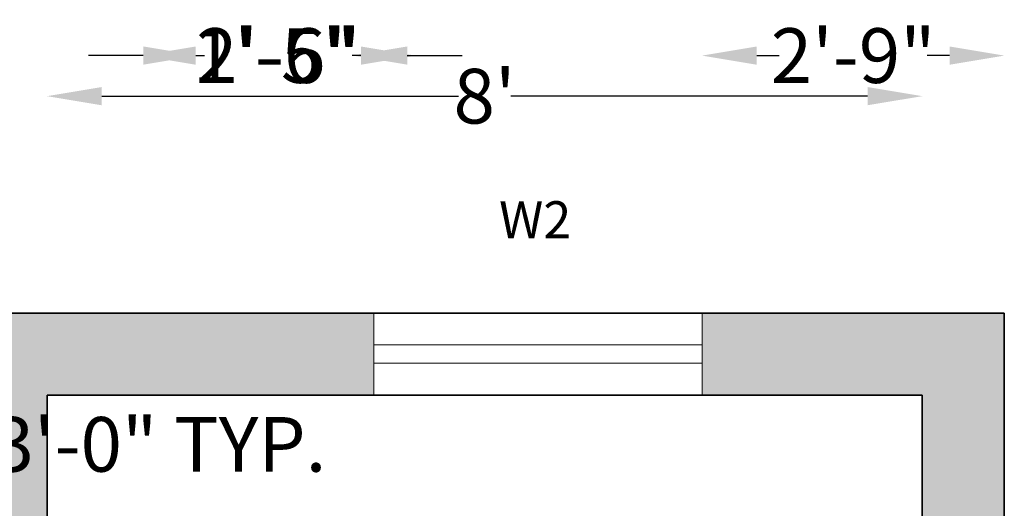
# Model space of a CAD drawing. Units: inches. Extents: x 2178 to 3409, y 1711 to 2279.
# Tile 7 of 8: x 2368 to 2476, y 2226 to 2279. Entities that reach past the tile are written whole.
import ezdxf

# ---------------------------------------------------------------- set-up
doc = ezdxf.new("R2010")
doc.units = ezdxf.units.IN
for name, color, linetype, lineweight in [('A-ANNO-DIMS', 2, 'Continuous', 18), ('A-ANNO-IDEN', 3, 'Continuous', 18), ('A-GLAZ', 4, 'Continuous', 18), ('A-WALL', 7, 'Continuous', 35), ('A-WALL-PATT', 252, 'Continuous', 13)]:
    doc.layers.add(name, color=color, linetype=linetype, lineweight=lineweight)
doc.styles.get("Standard").update_dxf_attribs({"font": 'arial.ttf'})
doc.dimstyles.get("Standard").update_dxf_attribs({"dimtxt": 6, "dimasz": 6, "dimexe": 0.18, "dimexo": 0.0625, "dimgap": 0.09, "dimtad": 0, "dimtih": 1, "dimtoh": 1, "dimdec": 4, "dimzin": 0, "dimdsep": 46, "dimlunit": 4, "dimtxsty": 'Standard', "dimcen": 0.09, "dimse1": 1, "dimse2": 1, "dimadec": 0, "dimazin": 0, "dimtfac": 1, "dimtdec": 4, "dimtofl": 0, "dimtmove": 0, "dimatfit": 3, "dimfxl": 1, "dimtolj": 1, "dimtzin": 0, "dimarcsym": 0})

# ---------------------------------------------------------------- blocks, each defined once
blk = doc.blocks.new('*D20')
at = {"layer": 'A-ANNO-DIMS', "color": 0, "lineweight": -2, "transparency": 16777216}
for p, q in [((2377.06, 2270.84), (2416.21, 2270.84)), ((2461.06, 2270.84), (2421.92, 2270.84))]:
    blk.add_line(p, q, dxfattribs=at)
at = {"layer": 'A-ANNO-DIMS', "color": 0, "transparency": 16777216}
for points in [[(2377.06, 2271.84), (2377.06, 2269.84), (2371.06, 2270.84)], [(2461.06, 2271.84), (2461.06, 2269.84), (2467.06, 2270.84)]]:
    blk.add_solid(points, dxfattribs=at)
at = {"layer": 'Defpoints', "color": 0, "transparency": 16777216}
for p in [(2467.06, 2270.84), (2371.06, 2238.04), (2467.06, 2238.04)]:
    blk.add_point(p, dxfattribs=at)
at = {"layer": 'A-ANNO-DIMS', "color": 0, "transparency": 16777216, "insert": (2419.06, 2270.84), "char_height": 6, "attachment_point": 5}
blk.add_mtext("\\A1;8'", dxfattribs=at)
blk = doc.blocks.new('*D21')
at = {"layer": 'A-ANNO-DIMS', "color": 0, "lineweight": -2, "transparency": 16777216}
for p, q in [((2502.61, 2232.04), (2502.61, 2175.14)), ((2502.61, 2112.04), (2502.61, 2168.94))]:
    blk.add_line(p, q, dxfattribs=at)
at = {"layer": 'A-ANNO-DIMS', "color": 0, "transparency": 16777216}
for points in [[(2501.61, 2232.04), (2503.61, 2232.04), (2502.61, 2238.04)], [(2501.61, 2112.04), (2503.61, 2112.04), (2502.61, 2106.04)]]:
    blk.add_solid(points, dxfattribs=at)
at = {"layer": 'Defpoints', "color": 0, "transparency": 16777216}
for p in [(2467.06, 2238.04), (2467.06, 2106.04), (2502.61, 2106.04)]:
    blk.add_point(p, dxfattribs=at)
at = {"layer": 'A-ANNO-DIMS', "color": 0, "transparency": 16777216, "insert": (2502.61, 2172.04), "char_height": 6, "attachment_point": 5}
blk.add_mtext("\\A1;11'", dxfattribs=at)
blk = doc.blocks.new('WINDOW-36')
for p, q in [((36, 9), (0, 9)), ((0, 9), (0, 0)), ((36, 0), (36, 9)), ((0, 5.5), (36, 5.5)), ((0, 3.5), (36, 3.5)), ((0, 0), (36, 0))]:
    blk.add_line(p, q)
blk = doc.blocks.new('*D47')
at = {"layer": 'A-ANNO-DIMS', "color": 0, "lineweight": -2, "transparency": 16777216}
for p, q in [((2291.22, 2232.64), (2315.22, 2232.64)), ((2321.22, 2232.64), (2327.22, 2232.64))]:
    blk.add_line(p, q, dxfattribs=at)
at = {"layer": 'A-ANNO-DIMS', "color": 0, "transparency": 16777216}
for points in [[(2291.22, 2233.64), (2291.22, 2231.64), (2285.22, 2232.64)], [(2315.22, 2233.64), (2315.22, 2231.64), (2321.22, 2232.64)]]:
    blk.add_solid(points, dxfattribs=at)
at = {"layer": 'Defpoints', "color": 0, "transparency": 16777216}
for p in [(2285.22, 2238.04), (2321.22, 2238.04), (2321.22, 2232.64)]:
    blk.add_point(p, dxfattribs=at)
at = {"layer": 'A-ANNO-DIMS', "color": 0, "transparency": 16777216, "insert": (2365.28, 2232.64), "char_height": 6, "attachment_point": 5}
blk.add_mtext('\\A1;WINDOW 3\'-0" TYP.', dxfattribs=at)
blk = doc.blocks.new('*D65')
at = {"layer": 'A-ANNO-DIMS', "color": 0, "lineweight": -2, "transparency": 16777216}
for p, q in [((2448.91, 2275.29), (2451.37, 2275.29)), ((2470.06, 2275.29), (2467.61, 2275.29))]:
    blk.add_line(p, q, dxfattribs=at)
at = {"layer": 'A-ANNO-DIMS', "color": 0, "transparency": 16777216}
for points in [[(2448.91, 2276.29), (2448.91, 2274.29), (2442.91, 2275.29)], [(2470.06, 2276.29), (2470.06, 2274.29), (2476.06, 2275.29)]]:
    blk.add_solid(points, dxfattribs=at)
at = {"layer": 'Defpoints', "color": 0, "transparency": 16777216}
for p in [(2476.06, 2275.29), (2442.91, 2247.04), (2476.06, 2247.04)]:
    blk.add_point(p, dxfattribs=at)
at = {"layer": 'A-ANNO-DIMS', "color": 0, "transparency": 16777216, "insert": (2459.49, 2275.29), "char_height": 6, "attachment_point": 5}
blk.add_mtext('\\A1;2\'-9"', dxfattribs=at)
blk = doc.blocks.new('*D71')
at = {"layer": 'A-ANNO-DIMS', "color": 0, "lineweight": -2, "transparency": 16777216}
for p, q in [((2381.625685, 2275.292563), (2375.625685, 2275.292563)), ((2410.582731, 2275.292563), (2416.582731, 2275.292563))]:
    blk.add_line(p, q, dxfattribs=at)
at = {"layer": 'A-ANNO-DIMS', "color": 0, "transparency": 16777216}
for points in [[(2381.625685, 2276.292563), (2381.625685, 2274.292563), (2387.625685, 2275.292563)], [(2410.582731, 2276.292563), (2410.582731, 2274.292563), (2404.582731, 2275.292563)]]:
    blk.add_solid(points, dxfattribs=at)
at = {"layer": 'Defpoints', "color": 0, "transparency": 16777216}
for p in [(2404.582731, 2275.292563), (2387.625685, 1942.827852), (2404.582731, 1942.827852)]:
    blk.add_point(p, dxfattribs=at)
at = {"layer": 'A-ANNO-DIMS', "color": 0, "transparency": 16777216, "insert": (2396.104208, 2275.292563), "char_height": 6, "attachment_point": 5}
blk.add_mtext('\\A1;1\'-5"', dxfattribs=at)
blk = doc.blocks.new('*D73')
at = {"layer": 'A-ANNO-DIMS', "color": 0, "lineweight": -2, "transparency": 16777216}
for p, q in [((2387.37, 2275.29), (2388.32, 2275.29)), ((2405.5, 2275.29), (2404.55, 2275.29))]:
    blk.add_line(p, q, dxfattribs=at)
at = {"layer": 'A-ANNO-DIMS', "color": 0, "transparency": 16777216}
for points in [[(2387.37, 2276.29), (2387.37, 2274.29), (2381.37, 2275.29)], [(2405.5, 2276.29), (2405.5, 2274.29), (2411.5, 2275.29)]]:
    blk.add_solid(points, dxfattribs=at)
at = {"layer": 'Defpoints', "color": 0, "transparency": 16777216}
for p in [(2411.5, 2275.29), (2381.37, 1966.49), (2411.5, 1966.49)]:
    blk.add_point(p, dxfattribs=at)
at = {"layer": 'A-ANNO-DIMS', "color": 0, "transparency": 16777216, "insert": (2396.44, 2275.29), "char_height": 6, "attachment_point": 5}
blk.add_mtext('\\A1;2\'-6"', dxfattribs=at)

msp = doc.modelspace()

# ---------------------------------------------------------------- hatches: boundary and pattern name
at = {"layer": 'A-WALL-PATT'}
h = msp.add_hatch(color=256, dxfattribs=at)
h.dxf.hatch_style = 1
h.paths.add_polyline_path([(2233.06485, 1992.04256), (2317.06485, 1992.04256), (2317.06485, 1998.04256), (2317.06485, 2006.75072), (2311.06485, 2006.75072), (2311.06485, 1998.04256), (2233.06485, 1998.04256), (2233.06485, 2009.64251), (2224.06485, 2009.64251), (2224.06485, 1863.04256), (2233.06485, 1863.04256), (2278.65041, 1863.04256), (2278.65041, 1872.04256), (2233.06485, 1872.04256)])
h.paths.add_polyline_path([(2359.06485, 1992.04256), (2359.06485, 1998.04256), (2353.06485, 1998.04256), (2353.06485, 1962.04256), (2353.06485, 1872.04256), (2314.65041, 1872.04256), (2314.65041, 1863.04256), (2359.06485, 1863.04256), (2359.06485, 1872.04256)])
h.paths.add_polyline_path([(2401.06485, 1890.04256), (2371.06485, 1890.04256), (2359.06485, 1890.04256), (2359.06485, 1884.04256), (2371.06485, 1884.04256), (2377.06485, 1884.04256), (2401.06485, 1884.04256)])
h.paths.add_polyline_path([(2353.06485, 1802.77269), (2359.06485, 1802.77269), (2359.06485, 1808.77269), (2356.83755, 1808.77269), (2353.06485, 1808.77269), (2347.91295, 1808.77269), (2347.91295, 1802.77269), (2347.91295, 1749.04256), (2342.02347, 1749.04256), (2342.02347, 1743.04256), (2353.06485, 1743.04256)])
h.paths.add_polyline_path([(2476.06485, 2247.04256), (2442.91353, 2247.04256), (2442.91353, 2238.04256), (2467.06485, 2238.04256), (2467.06485, 2041.93675), (2476.06485, 2041.93675)])
h.paths.add_polyline_path([(2467.06485, 2106.04256), (2406.56133, 2106.04256, -0.04188649), (2407.06485, 2100.04256), (2467.06485, 2100.04256)])
h.paths.add_polyline_path([(2406.91353, 2247.04256), (2321.22384, 2247.04256), (2321.22384, 2238.04256), (2365.06485, 2238.04256), (2365.06485, 2106.04256), (2365.06485, 2100.04256), (2371.06485, 2100.04256), (2371.06485, 2136.04256), (2371.06485, 2238.04256), (2406.91353, 2238.04256)])
h.paths.add_polyline_path([(2285.22384, 2247.04256), (2224.06485, 2247.04256), (2224.06485, 2087.1459), (2233.06485, 2087.1459), (2233.06485, 2100.04256), (2329.06485, 2100.04256, -0.04188649), (2329.56837, 2106.04256), (2233.06485, 2106.04256), (2233.06485, 2238.04256), (2285.22384, 2238.04256)])
h.paths.add_polyline_path([(2317.06485, 2052.04256), (2317.06485, 2061.5418), (2311.06485, 2061.5418), (2311.06485, 2052.04256), (2233.06485, 2052.04256), (2233.06485, 2063.1459), (2224.06485, 2063.1459), (2224.06485, 2033.64251), (2233.06485, 2033.64251), (2233.06485, 2046.04256), (2311.06485, 2046.04256), (2311.06485, 2036.1446, -0.050382044), (2317.06485, 2036.75072), (2317.06485, 2046.04256)])

# ---------------------------------------------------------------- linework, layer by layer
at = {"layer": 'A-WALL'}
for p, q in [((2224.06485, 2247.04256), (2476.06485, 2247.04256)), ((2476.06485, 2247.04256), (2476.06485, 1803.04256)), ((2371.06485, 2238.04256), (2371.06485, 2106.04256)), ((2371.06485, 2238.04256), (2467.06485, 2238.04256)), ((2467.06485, 2238.04256), (2467.06485, 1812.04256))]:
    msp.add_line(p, q, dxfattribs=at)

# ---------------------------------------------------------------- block references
at = {"layer": 'A-GLAZ'}
msp.add_blockref('WINDOW-36', (2406.91353, 2238.04256), dxfattribs=at)

# ---------------------------------------------------------------- texts
at = {"layer": 'A-ANNO-IDEN', "insert": (2420.6445, 2259.31141), "char_height": 4.051205, "attachment_point": 1}
msp.add_mtext_dynamic_manual_height_columns('W2', width=167.0263497, gutter_width=20.25603, heights=[0], dxfattribs=at)

# ---------------------------------------------------------------- dimensions: what is measured, and where the dimension line sits
at = {"layer": 'A-ANNO-DIMS'}
for base, p1, p2, override, picture, middle in [((2404.58273, 2275.29256), (2387.62568, 1942.82785), (2404.58273, 1942.82785), {"dimdec": 1, "dimlfac": 1, "dimrnd": 0, "dimzin": 1, "dimdsep": 46, "dimlunit": 4, "dimfrac": 2}, '*D71', (2396.10421, 2275.29256)), ((2411.50157, 2275.29256), (2381.37394, 1966.48789), (2411.50157, 1966.48789), {"dimdec": 1, "dimlfac": 1, "dimrnd": 0, "dimzin": 1, "dimdsep": 46, "dimlunit": 4, "dimfrac": 2}, '*D73', (2396.43775, 2275.29256)), ((2476.06485, 2275.29256), (2442.91353, 2247.04256), (2476.06485, 2247.04256), {"dimdec": 1, "dimlfac": 1, "dimrnd": 0, "dimzin": 1, "dimdsep": 46, "dimlunit": 4, "dimfrac": 2}, '*D65', (2459.48919, 2275.29256)), ((2467.06485, 2270.8418), (2371.06485, 2238.04256), (2467.06485, 2238.04256), {"dimclrd": 0, "dimclre": 0, "dimclrt": 0}, '*D20', (2419.06485, 2270.8418))]:
    dim = msp.add_linear_dim(base=base, p1=p1, p2=p2, dimstyle='Standard', override=override, dxfattribs=at)
    dim.commit()
    dim.dimension.update_dxf_attribs({"geometry": picture, "text_midpoint": middle})
dim = msp.add_linear_dim(base=(2321.22384, 2232.64256), p1=(2285.22384, 2238.04256), p2=(2321.22384, 2238.04256), text='WINDOW <> TYP.', dimstyle='Standard', override={"dimdec": 1, "dimlfac": 1, "dimrnd": 0, "dimzin": 1, "dimdsep": 46, "dimlunit": 4, "dimfrac": 2}, dxfattribs=at)
dim.commit()
dim.dimension.update_dxf_attribs({"geometry": '*D47', "text_midpoint": (2365.27632, 2232.64256)})
dim = msp.add_linear_dim(base=(2502.61341, 2106.04256), p1=(2467.06485, 2238.04256), p2=(2467.06485, 2106.04256), angle=90, dimstyle='Standard', override={"dimclrd": 0, "dimclre": 0, "dimclrt": 0}, dxfattribs=at)
dim.commit()
dim.dimension.update_dxf_attribs({"geometry": '*D21', "text_midpoint": (2502.61341, 2172.04256)})

doc.saveas('drawing.dxf')
